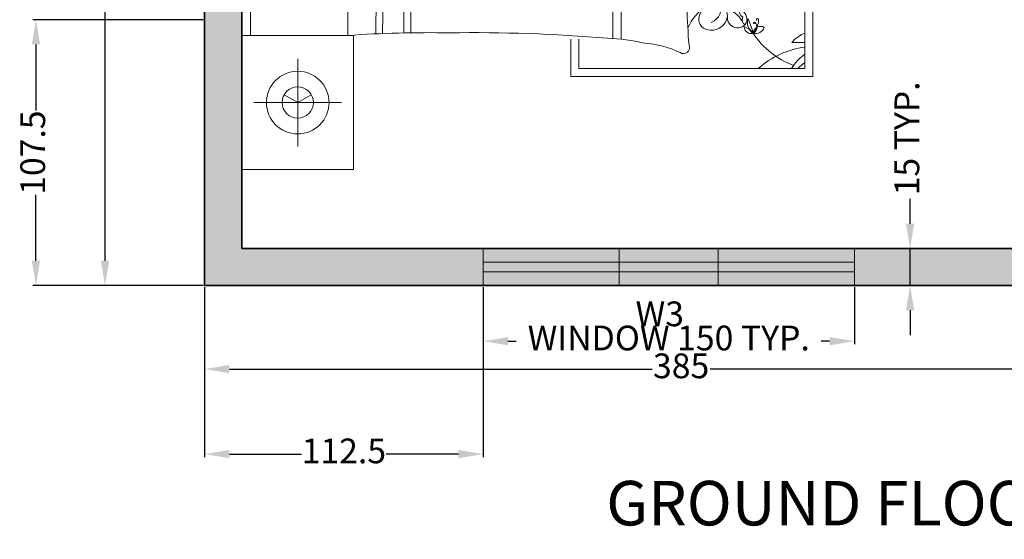
# Model space of a CAD drawing. Units: centimetres. Extents: x 2401 to 3632, y 2122 to 3526.
# Tile 1 of 10: x 2426 to 2824, y 2163 to 2374. Entities that reach past the tile are written whole.
import ezdxf

# ---------------------------------------------------------------- set-up
doc = ezdxf.new("R2010")
doc.units = ezdxf.units.CM
for name, color, linetype, lineweight in [('A-ANNO-DIMS', 9, 'Continuous', 18), ('A-ANNO-TEXT', 9, 'Continuous', 18), ('A-FURN', 9, 'Continuous', 18), ('A-GLAZ', 4, 'Continuous', 18), ('A-WALL', 7, 'Continuous', 35)]:
    doc.layers.add(name, color=color, linetype=linetype, lineweight=lineweight)
doc.layers.add('A-GLAZ-PATT', color=251, linetype='Continuous', lineweight=13, true_color=0x636466)
doc.layers.add('A-WALL-PATT', color=18, linetype='Continuous', lineweight=13, true_color=0x000000)
doc.styles.get("Standard").update_dxf_attribs({"font": 'arial.ttf'})
doc.dimstyles.new('ISO-25', dxfattribs={"dimtxt": 10, "dimasz": 10, "dimexe": 1.25, "dimexo": 0.625, "dimtad": 0, "dimtxsty": 'Standard', "dimcen": 2.5, "dimadec": 0, "dimazin": 0, "dimtfac": 1, "dimtmove": 0, "dimatfit": 3, "dimfxl": 1, "dimarcsym": 0})

# ---------------------------------------------------------------- blocks, each defined once
blk = doc.blocks.new('bed')
for p, q in [((3025.77, 3949.95), (3025.77, 3649.95)), ((3000.77, 3900.35), (3000.77, 3939.55)), ((2981.17, 3919.95), (3020.37, 3919.95)), ((2770.64, 3910.36), (2878.71, 3910.36)), ((2770.64, 3691.65), (2770.64, 3910.36)), ((2774.11, 3906.88), (2774.11, 3695.12)), ((2875.23, 3906.88), (2774.11, 3906.88)), ((2875.23, 3893.39), (2875.23, 3906.88)), ((2878.71, 3910.36), (2878.71, 3893.39)), ((2856.25, 3708.31), (2856.25, 3893.41)), ((2860, 3708.59), (2860, 3893.41)), ((2937.86, 3890.21), (2940.29, 3892.64)), ((2939.08, 3878.06), (2937.86, 3890.21)), ((2940.29, 3892.64), (2953.05, 3881.7)), ((3025.77, 3889.95), (2943.43, 3889.95)), ((2978.36, 3889.95), (2978.36, 3709.95)), ((3021.92, 3709.95), (3021.92, 3889.95)), ((2953.05, 3881.7), (2961.55, 3870.16)), ((2804.53, 3877.32), (2807.92, 3877.98)), ((2937.86, 3862.87), (2939.08, 3878.06)), ((2961.55, 3870.16), (2969.44, 3848.28)), ((2936.04, 3849.5), (2937.86, 3862.87)), ((2826.78, 3739.05), (2826.78, 3860.86)), ((2804.53, 3856.35), (2807.92, 3855.69)), ((2932.4, 3841.6), (2936.04, 3849.5)), ((2969.44, 3848.28), (2978.36, 3815.57)), ((2929.97, 3831.88), (2932.4, 3841.6)), ((2937.86, 3830.66), (2929.97, 3831.88)), ((2955.47, 3823.98), (2937.86, 3830.66)), ((2950.29, 3711.02), (2949.82, 3826.13)), ((2953.37, 3711.03), (2952.92, 3824.95)), ((2978.36, 3807.54), (2955.47, 3823.98)), ((2962.82, 3710.88), (2961.28, 3819.81)), ((2965.89, 3710.76), (2964.4, 3817.57)), ((2804.53, 3745.65), (2807.92, 3746.31)), ((2804.53, 3724.68), (2807.92, 3724.02)), ((2875.23, 3695.12), (2875.23, 3708.35)), ((2878.71, 3708.28), (2878.71, 3691.65)), ((3000.77, 3699.55), (3000.77, 3660.35)), ((2878.71, 3691.65), (2770.64, 3691.65)), ((2774.11, 3695.12), (2875.23, 3695.12)), ((2981.17, 3679.95), (3020.37, 3679.95))]:
    blk.add_line(p, q)
for points in [[(2975.77, 3889.95), (2975.77, 3949.95), (3025.77, 3949.95)], [(3000.77, 3919.95), (2994.7, 3916.45)], [(3000.77, 3919.95), (3006.83, 3916.45)], [(3025.77, 3709.95), (2975.77, 3709.95), (2975.77, 3649.95), (3025.77, 3649.95)], [(3000.77, 3679.95), (2994.7, 3683.45)], [(3000.77, 3679.95), (3006.83, 3683.45)]]:
    blk.add_lwpolyline(points)
for points in [[(2912.82, 3893.27, 0.001242), (2855.9, 3893.41, -0.127202), (2827.53, 3899.43)], [(3018.29, 3872.72, 0.074897), (2998.69, 3872.36, -0.472817)], [(2997.6, 3801.36, 0.14099), (3017.59, 3800.76, 0.235245)], [(2997.6, 3788.55, -0.14099), (3017.59, 3789.15, -0.235245)], [(3018.29, 3727.19, -0.074897), (2998.69, 3727.55, 0.472817)], [(2862.36, 3708.67, 0.056112), (2845.85, 3706.5, 0.095341), (2829.95, 3702.28)]]:
    blk.add_lwpolyline(points, format="xyb")
for centre, radius in [((3000.77, 3919.95), 14), ((3000.77, 3919.95), 7), ((2785.6, 3864.98), 0.764), ((2793.66, 3859.99), 0.764), ((2793.66, 3742.02), 0.764), ((2785.6, 3737.02), 0.764), ((3000.77, 3679.95), 14), ((3000.77, 3679.95), 7)]:
    blk.add_circle(centre, radius)
for centre, radius, start, end in [((2760.03, 3923.26), 23.79, 306.3036, 316.4814), ((2763.59, 3916.39), 19.09, 303.4617, 330.1116), ((2768.83, 3936.05), 39.18, 277.745, 311.8856), ((2764.96, 3869.02), 39.18, 34.3865, 68.5908), ((2827.73, 3896.66), 2.77, 93.98, 207.3412), ((2768, 3905.7), 15.93, 292.5547, 318.9546), ((2776.56, 3949.33), 54.2, 267.4081, 273.6519), ((2514.5, 3864.44), 312.3, 359.3433, 5.6887), ((2796.37, 3886.9), 4.34, 77.7115, 159.0387), ((2794.02, 3891.25), 3.27, 238.4633, 358.2869), ((2804.75, 3884.63), 9.91, 138.8402, 177.9352), ((2798.78, 3888.31), 3.2, 117.6827, 223.7762), ((2798.06, 3887.99), 3.25, 2.9516, 103.728), ((2824.04, 3897.09), 27.41, 192.5173, 207.1824), ((2793.67, 3886.12), 6.19, 345.4653, 54.2343), ((2803, 3894.63), 6.69, 211.3827, 255.2969), ((2815.84, 3882.53), 7.17, 84.9449, 172.8857), ((2816.56, 3884.61), 5.07, 354.4856, 91.0538), ((2932.84, 4167.71), 275.17, 265.8294, 271.553), ((3046.53, 3887.51), 113.22, 177.4519, 191.3392), ((2795.33, 3884.97), 0.487, 177.9352, 11.4834), ((2795.58, 3885.02), 0.236, 11.4834, 127.9409), ((2796.77, 3886.39), 0.424, 223.7762, 159.7183), ((2805.64, 3885.26), 5.62, 175.969, 254.3045), ((2804.28, 3884.18), 4.5, 350.264, 160.8688), ((2799.41, 3885.11), 2.76, 333.9755, 53.2681), ((2814.2, 3893.11), 14.16, 211.2614, 251.7045), ((2818.55, 3879.71), 6.96, 111.5819, 201.4221), ((2805.66, 3897.83), 22.71, 303.6671, 333.2997), ((2798.17, 3879.2), 5.99, 6.1662, 51.5825), ((2817.43, 3883.78), 8.71, 182.3591, 234.0401), ((2812.81, 3886.16), 9.02, 265.2933, 346.921), ((2813.05, 3893.24), 16.1, 236.2883, 266.5076), ((2810.99, 3881.04), 7.46, 209.9085, 343.1337), ((2814.13, 3876.31), 1.86, 167.3041, 285.1471), ((2819.17, 3867.4), 11.57, 122.7011, 126.3445), ((2821.34, 3879.88), 9.56, 199.2822, 299.1751), ((2824.57, 3889.51), 12.43, 238.8218, 279.1554), ((2819.17, 3867.4), 11.57, 55.785, 94.7304), ((2823.47, 3874.11), 3.61, 30.0293, 52.325), ((2789.51, 3870.54), 0.853, 56.8636, 146.9021), ((2801.41, 3872.25), 8.46, 178.3264, 187.1302), ((2792.27, 3871.07), 1.58, 11.3256, 64.4621), ((2797.62, 3873.34), 4.74, 190.2588, 210.656), ((2797.6, 3874.36), 4.82, 218.2101, 226.3071), ((2775.06, 3890.75), 28.48, 313.1541, 322.0459), ((2796.01, 3873.64), 0.586, 142.4737, 265.053), ((2796.78, 3873.76), 1.26, 127.7621, 169.0403), ((2796.11, 3874.82), 1.78, 265.053, 338.3618), ((2798.46, 3872.39), 2.32, 113.4276, 137.6104), ((2798.2, 3874.8), 0.764, 183.2768, 356.7232), ((2798.76, 3873.41), 1.25, 139.7889, 227.6792), ((2798.36, 3872.98), 0.658, 227.6792, 350.3487), ((2795.81, 3873.43), 2.5, 353.0852, 15.7171), ((2797.45, 3873.13), 1.58, 350.3487, 43.6538), ((2800.38, 3874.76), 1.84, 198.7263, 262.5032), ((2798.92, 3873.91), 0.73, 1.1081, 91.8675), ((2800.29, 3873.51), 0.59, 255.2356, 54.9248), ((2799.38, 3873.74), 1.27, 11.5637, 52.6358), ((2816.22, 3868.58), 6.15, 41.5653, 105.1471), ((2819.61, 3881.32), 8.62, 277.436, 299.9149), ((2824.18, 3875.64), 4.49, 221.5653, 293.8354), ((2823.47, 3874.11), 3.61, 314.4517, 333.558), ((3021.8, 3862.02), 40.2, 165.1039, 191.0369), ((2990.83, 3834.5), 38.67, 65.1316, 101.7583), ((5873.3, 3707.37), 2859.79, 176.68521, 177.14978), ((2785.02, 3866.54), 1.51, 157.4086, 261.4386), ((2784.17, 3866.59), 0.757, 58.0499, 135.6268), ((2783.3, 3865.19), 2.41, 14.7558, 58.0499), ((2786.72, 3869.91), 0.853, 124.3538, 214.3923), ((2787.97, 3869.78), 1.99, 190.3057, 287.1958), ((2788.54, 3870.49), 2.31, 176.9701, 248.2913), ((2805.02, 3882.67), 22.32, 212.6784, 216.3746), ((2787.76, 3869.95), 0.883, 216.3746, 291.7548), ((2795.58, 3857.56), 12.46, 124.0033, 132.4917), ((2782.77, 3855.98), 13.31, 63.7819, 68.2913), ((2789.87, 3866.22), 2.12, 128.3208, 208.8162), ((2789.87, 3869.34), 1.99, 122.8155, 187.3992), ((2788.34, 3868.51), 0.666, 289.3605, 111.7548), ((2788.84, 3868.51), 0.666, 221.8703, 44.2646), ((2791.86, 3866.57), 3.48, 157.2305, 229.0635), ((2790.75, 3869.08), 2.31, 109.4799, 177.6828), ((2790.69, 3867.72), 2.05, 174.4544, 220.6188), ((2779.03, 3856.28), 14.94, 30.544, 49.818), ((2789.95, 3869.59), 0.883, 148.8844, 224.2646), ((2808.3, 3858.51), 22.32, 145.1882, 148.8844), ((2795.58, 3857.56), 12.46, 94.756, 119.2041), ((2822.1, 3839.62), 40.99, 132.2412, 142.1744), ((2794.44, 3871.41), 1.44, 188.3432, 274.2869), ((2795.7, 3872.2), 2.51, 210.656, 242.6341), ((2794.04, 3870.31), 0.611, 325.7657, 67.4417), ((2796.2, 3845.18), 24.85, 73.5842, 93.8277), ((2811.5, 3870.46), 8.46, 178.3264, 187.1302), ((2802.37, 3869.29), 1.58, 11.3256, 64.4621), ((2807.71, 3871.55), 4.74, 190.2588, 210.656), ((2804.53, 3869.62), 1.44, 188.3432, 274.2869), ((2805.8, 3870.42), 2.51, 210.656, 242.6341), ((2807.7, 3872.58), 4.82, 218.2101, 226.3071), ((2804.13, 3868.53), 0.611, 325.7657, 67.4417), ((2805.85, 3867.41), 1.44, 147.5332, 233.4768), ((2804.7, 3867.58), 0.611, 354.3784, 96.0543), ((2807.15, 3868.15), 2.51, 179.1859, 211.164), ((2796.2, 3845.18), 24.85, 63.0032, 69.8941), ((2809.96, 3868.8), 4.82, 195.5129, 203.6099), ((2783.42, 3863.83), 0.586, 142.4737, 265.053), ((2784.19, 3863.94), 1.26, 61.2196, 169.0403), ((2783.52, 3865.01), 1.78, 265.053, 338.3618), ((2785.87, 3862.58), 2.32, 113.4276, 137.6104), ((2784.96, 3866.11), 0.506, 172.906, 277.132), ((2786.17, 3863.6), 1.25, 139.7889, 227.6792), ((2785.77, 3863.16), 0.658, 227.6792, 350.3487), ((2786.67, 3865.83), 1.04, 36.1046, 181.4281), ((2783.22, 3863.62), 2.5, 353.0852, 15.7171), ((2784.86, 3863.32), 1.58, 350.3487, 43.6538), ((2787.79, 3864.95), 1.84, 198.7263, 262.5032), ((2786.06, 3866.65), 1.05, 270.0645, 331.1507), ((2786.96, 3866.4), 1.2, 221.8413, 265.7877), ((2786.33, 3864.09), 0.73, 1.1081, 91.8675), ((2786.95, 3865.94), 0.749, 263.7526, 41.7054), ((2786.79, 3863.93), 1.27, 11.5637, 86.365), ((2787.7, 3863.7), 0.59, 255.2356, 54.9248), ((2790.26, 3866.38), 2.53, 207.7043, 254.3516), ((2788.61, 3864.93), 3.48, 270.278, 342.111), ((2790.93, 3860.58), 2.46, 98.7227, 159.3375), ((2787.26, 3864.79), 2.46, 340.0041, 40.6188), ((2790.25, 3865.04), 2.05, 278.7227, 324.8872), ((2789.89, 3863.37), 2.12, 290.5253, 358.5375), ((2794.02, 3863.97), 2.12, 182.8499, 266.1226), ((2793.19, 3865.47), 2.05, 231.7607, 277.9252), ((2794.79, 3865.83), 3.48, 214.5369, 286.3699), ((2793.81, 3861), 2.46, 37.3105, 97.9252), ((2809.06, 3869.3), 4.74, 211.164, 231.5612), ((2809.89, 3873.16), 8.46, 234.6898, 243.4936), ((2804.54, 3865.66), 1.58, 357.3579, 50.4944), ((2811.3, 3865.97), 0.578, 12.7051, 190.4384), ((2811.66, 3866.04), 0.94, 190.4384, 10.4136), ((2821.34, 3853.79), 9.56, 60.8249, 160.7178), ((2911.57, 3860.44), 24.42, 336.2616, 11.3392), ((2789.7, 3863.74), 2.53, 244.9899, 291.6373), ((2791.47, 3858.83), 0.586, 142.4737, 265.053), ((2792.24, 3858.95), 1.26, 61.2196, 169.0403), ((2791.57, 3860.01), 1.78, 265.053, 338.3618), ((2793.07, 3861.54), 1.51, 157.4086, 261.4386), ((2792.22, 3861.59), 0.757, 58.0499, 135.6268), ((2793.92, 3857.58), 2.32, 113.4276, 137.6104), ((2793.01, 3861.12), 0.506, 172.906, 277.132), ((2791.35, 3860.19), 2.41, 14.7558, 58.0499), ((2779.03, 3856.28), 14.94, 23.0501, 23.8477), ((2794.22, 3858.6), 1.25, 139.7889, 227.6792), ((2794.72, 3860.83), 1.04, 36.1046, 181.4281), ((2791.27, 3858.62), 2.5, 353.0852, 15.7171), ((2794.09, 3864.38), 2.53, 265.0106, 311.658), ((2792.91, 3858.32), 1.58, 350.3487, 43.6538), ((2795.84, 3859.95), 1.84, 198.7263, 262.5032), ((2794.11, 3861.65), 1.05, 270.0645, 331.1507), ((2795.01, 3861.4), 1.2, 221.8413, 265.7877), ((2794.38, 3859.1), 0.73, 1.1081, 91.8675), ((2795, 3860.95), 0.749, 263.7526, 41.7054), ((2794.84, 3858.93), 1.27, 11.5637, 86.365), ((2795.75, 3858.7), 0.59, 255.2356, 54.9248), ((2810.99, 3852.63), 7.46, 16.8663, 150.0915), ((2814.13, 3857.35), 1.86, 74.8529, 192.6959), ((2816.22, 3865.09), 6.15, 254.8529, 318.4347), ((2819.61, 3852.35), 8.62, 60.0851, 82.564), ((2824.18, 3858.03), 4.49, 66.1646, 138.4347), ((2823.47, 3859.56), 3.61, 23.229, 45.5483), ((2793.82, 3858.17), 0.658, 227.6792, 350.3487), ((2779.03, 3856.28), 14.94, 357.1071, 4.7585), ((2805.64, 3848.41), 5.62, 105.6955, 184.031), ((2798.17, 3854.46), 5.99, 308.4175, 353.8338), ((2814.2, 3840.56), 14.16, 108.2955, 148.7386), ((2813.05, 3840.43), 16.1, 93.4924, 123.7117), ((2817.43, 3849.89), 8.71, 125.9599, 177.6409), ((2818.55, 3853.96), 6.96, 158.5779, 248.4181), ((2812.81, 3847.51), 9.02, 13.079, 94.7067), ((2819.17, 3866.26), 11.57, 233.6555, 237.2989), ((2824.57, 3844.16), 12.43, 79.7133, 121.1782), ((2819.17, 3866.26), 11.57, 265.2696, 304.215), ((2805.66, 3835.83), 22.71, 21.4941, 56.3329), ((2823.47, 3859.56), 3.61, 307.675, 336.7144), ((3050.38, 3840.86), 69.73, 168.0397, 199.2615), ((2804.28, 3849.49), 4.5, 199.1312, 9.736), ((2799.41, 3848.56), 2.76, 306.7319, 26.0245), ((2815.84, 3851.14), 7.17, 187.1143, 275.0551), ((2816.56, 3849.06), 5.07, 268.9462, 5.5144), ((3043.34, 3811.05), 116.34, 160.1194, 169.3383), ((2909.73, 3831.62), 108.8, 352.2196, 9.497), ((2794.02, 3842.42), 3.27, 1.7131, 121.5367), ((2796.37, 3846.77), 4.34, 200.9613, 282.2885), ((2795.33, 3848.7), 0.487, 348.5166, 182.0648), ((2804.75, 3849.04), 9.91, 182.0648, 221.1598), ((2795.58, 3848.65), 0.236, 232.0591, 348.5166), ((2798.78, 3845.36), 3.2, 136.2238, 242.3173), ((2796.93, 3847.24), 0.255, 200.2667, 136.2271), ((2793.67, 3847.55), 6.19, 305.7657, 14.5347), ((2824.04, 3836.58), 27.41, 152.8176, 167.4827), ((2798.06, 3845.68), 3.25, 256.272, 357.0484), ((2803, 3839.04), 6.69, 104.7031, 148.6173), ((2768, 3827.97), 15.93, 41.0454, 67.4453), ((2764.96, 3864.65), 39.18, 291.4092, 325.6135), ((2776.56, 3784.33), 54.2, 86.3481, 92.5919), ((2768.83, 3797.62), 39.18, 4.4623, 82.255), ((2763.59, 3817.28), 19.09, 1.272, 56.5383), ((2929.73, 3832.56), 0.724, 178.8623, 289.7536), ((2760.03, 3810.41), 23.79, 17.8504, 53.6964), ((2753.34, 3797.91), 35.39, 34.0123, 54.053), ((2747.85, 3800.62), 39.18, 4.4623, 27.4146), ((3035.15, 3812.63), 52.9, 169.8617, 193.6238), ((2964.72, 3808.64), 53.46, 351.5249, 13.96), ((2753.52, 3811.58), 21.54, 343.5431, 17.0202), ((2742.41, 3803.04), 31.85, 4.3787, 5.6357), ((2720.59, 3786.27), 56.92, 19.7217, 19.9028), ((2783.99, 3800.45), 4.34, 47.7873, 129.1145), ((2784.12, 3805.39), 3.27, 208.5391, 328.3627), ((2790.12, 3794.3), 9.91, 108.9159, 148.011), ((2786.78, 3800.47), 3.2, 87.7585, 193.852), ((2813.06, 3795.47), 27.41, 162.593, 177.2582), ((2781.26, 3801.12), 6.19, 315.5411, 24.3101), ((2793.6, 3803.84), 6.69, 181.4585, 225.3727), ((2786, 3800.55), 3.25, 333.0274, 73.8037), ((2804.97, 3797.45), 4.34, 47.7873, 129.1145), ((2987.57, 3836.72), 36.76, 264.0129, 285.8293), ((2782.13, 3799.29), 0.487, 148.011, 341.5592), ((2782.37, 3799.21), 0.236, 341.5592, 98.0167), ((2784.08, 3799.8), 0.424, 193.852, 129.9245), ((2805.11, 3802.39), 3.27, 208.5391, 328.3627), ((2811.1, 3791.3), 9.91, 108.9159, 148.011), ((2807.77, 3797.47), 3.2, 87.7585, 193.852), ((2805.07, 3796.8), 0.424, 193.852, 129.9245), ((2802.25, 3798.12), 6.19, 315.5411, 24.3101), ((2834.04, 3792.47), 27.41, 162.593, 177.2582), ((2802.25, 3793.88), 6.19, 335.6899, 44.4589), ((2834.04, 3799.53), 27.41, 182.7418, 197.407), ((2806.98, 3797.55), 3.25, 333.0274, 73.8037), ((2814.58, 3800.84), 6.69, 181.4585, 225.3727), ((2782.13, 3792.71), 0.487, 18.4408, 211.989), ((2790.12, 3797.71), 9.91, 211.989, 251.0841), ((2782.37, 3792.79), 0.236, 261.9833, 18.4408), ((2786.78, 3791.54), 3.2, 166.148, 272.2415), ((2784.25, 3792.24), 0.255, 230.1909, 166.0209), ((2813.06, 3796.53), 27.41, 182.7418, 197.407), ((2781.26, 3790.88), 6.19, 335.6899, 44.4589), ((2793.6, 3788.16), 6.69, 134.6273, 178.5415), ((2786, 3791.45), 3.25, 286.1963, 26.9726), ((2805.11, 3789.62), 3.27, 31.6373, 151.4609), ((2803.11, 3796.29), 0.487, 148.011, 341.5592), ((2803.11, 3795.71), 0.487, 18.4408, 211.989), ((2811.1, 3800.7), 9.91, 211.989, 251.0841), ((2803.35, 3796.21), 0.236, 341.5592, 98.0167), ((2803.35, 3795.79), 0.236, 261.9833, 18.4408), ((2807.77, 3794.53), 3.2, 166.148, 272.2415), ((2805.23, 3795.24), 0.255, 230.1909, 166.0209), ((2806.98, 3794.45), 3.25, 286.1963, 26.9726), ((2814.58, 3791.16), 6.69, 134.6273, 178.5415), ((2777.88, 3795.65), 30.32, 262.8636, 351.8197), ((2784.12, 3786.62), 3.27, 31.6373, 151.4609), ((2783.99, 3791.55), 4.34, 230.8855, 312.2127), ((2747.85, 3791.38), 39.18, 332.5854, 355.5377), ((2804.97, 3794.55), 4.34, 230.8855, 312.2127), ((2998.15, 3783.03), 15.9, 155.0183, 198.5407), ((2987.57, 3753.18), 36.76, 74.1707, 95.9871), ((3003.33, 3785.03), 14.84, 333.3437, 16.1026), ((2753.52, 3780.42), 21.54, 342.9798, 16.4569), ((2742.41, 3788.96), 31.85, 354.3643, 355.6213), ((2720.59, 3805.74), 56.92, 340.0972, 340.2783), ((2780.65, 3791.73), 17.54, 248.117, 276.6195), ((2775.77, 3775.64), 7.03, 256.3898, 349.0739), ((2776.73, 3780.92), 8.89, 252.8609, 311.9049), ((2764.96, 3737.36), 39.18, 34.3865, 68.5908), ((3018.84, 3755.24), 38.19, 153.8761, 196.1746), ((2965.8, 3762.79), 52.74, 346.3427, 11.1841), ((2776.56, 3817.67), 54.2, 267.4081, 273.6519), ((2768, 3774.04), 15.93, 292.5547, 318.9546), ((2796.37, 3755.24), 4.34, 77.7115, 159.0387), ((2794.02, 3759.58), 3.27, 238.4633, 358.2869), ((2804.75, 3752.96), 9.91, 138.8402, 177.9352), ((2798.78, 3756.64), 3.2, 117.6827, 223.7762), ((2798.06, 3756.33), 3.25, 2.9516, 103.728), ((2803, 3762.97), 6.69, 211.3827, 255.2969), ((2793.67, 3754.46), 6.19, 345.4653, 54.2343), ((2824.04, 3765.42), 27.41, 192.5173, 207.1824), ((2804.28, 3752.51), 4.5, 350.264, 160.8688), ((2815.84, 3750.86), 7.17, 84.9449, 172.8857), ((2816.56, 3752.94), 5.07, 354.4856, 91.0538), ((2805.66, 3766.17), 22.71, 303.6671, 338.5059), ((2795.33, 3753.3), 0.487, 177.9352, 11.4834), ((2795.58, 3753.35), 0.236, 11.4834, 127.9409), ((2796.77, 3754.72), 0.424, 223.7762, 159.7183), ((2805.64, 3753.59), 5.62, 175.969, 254.3045), ((2799.41, 3753.44), 2.76, 333.9755, 53.2681), ((2814.2, 3761.44), 14.16, 211.2614, 251.7045), ((2818.55, 3748.05), 6.96, 111.5819, 201.4221), ((2798.17, 3747.54), 5.99, 6.1662, 51.5825), ((2813.05, 3761.57), 16.1, 236.2883, 266.5076), ((2817.43, 3752.11), 8.71, 182.3591, 234.0401), ((2812.81, 3754.5), 9.02, 265.2933, 346.921), ((5873.3, 3892.54), 2859.79, 182.85022, 183.31479), ((2794.22, 3743.4), 1.25, 132.3208, 220.2111), ((2793.82, 3743.84), 0.658, 9.6513, 132.3208), ((2779.03, 3745.73), 14.94, 355.2415, 2.8929), ((2792.91, 3743.68), 1.58, 316.3462, 9.6513), ((2795.84, 3742.05), 1.84, 97.4968, 161.2737), ((2795.75, 3743.3), 0.59, 305.0752, 104.7644), ((2810.99, 3749.37), 7.46, 209.9085, 343.1337), ((2814.13, 3744.65), 1.86, 167.3041, 285.1471), ((2819.17, 3735.74), 11.57, 122.7011, 126.3445), ((2821.34, 3748.21), 9.56, 199.2822, 299.1751), ((2824.57, 3757.84), 12.43, 238.8218, 280.2867), ((2819.17, 3735.74), 11.57, 55.785, 94.7304), ((2823.47, 3742.45), 3.61, 23.2856, 52.325), ((3021.8, 3737.89), 40.2, 168.9631, 194.8961), ((2785.77, 3738.84), 0.658, 9.6513, 132.3208), ((2789.7, 3738.26), 2.53, 68.3627, 115.0101), ((2788.61, 3737.07), 3.48, 17.889, 89.722), ((2790.93, 3741.42), 2.46, 200.6625, 261.2773), ((2789.89, 3738.63), 2.12, 1.4625, 69.4747), ((2791.47, 3743.17), 0.586, 94.947, 217.5263), ((2792.24, 3743.06), 1.26, 190.9597, 298.7804), ((2791.57, 3741.99), 1.78, 21.6382, 94.947), ((2793.07, 3740.46), 1.51, 98.5614, 202.5914), ((2792.22, 3740.41), 0.757, 224.3732, 301.9501), ((2794.02, 3738.03), 2.12, 93.8774, 177.1501), ((2794.79, 3736.17), 3.48, 73.6301, 145.4631), ((2793.92, 3744.42), 2.32, 222.3896, 246.5724), ((2793.01, 3740.89), 0.506, 82.868, 187.094), ((2791.35, 3741.81), 2.41, 301.9501, 345.2442), ((2779.03, 3745.73), 14.94, 336.1523, 336.9499), ((2793.81, 3741), 2.46, 262.0748, 322.6895), ((2791.27, 3743.38), 2.5, 344.2829, 6.9148), ((2794.72, 3741.17), 1.04, 178.5719, 323.8954), ((2794.09, 3737.62), 2.53, 48.342, 94.9894), ((2795.01, 3740.6), 1.2, 94.2123, 138.1587), ((2794.11, 3740.35), 1.05, 28.8493, 89.9355), ((2794.38, 3742.91), 0.73, 268.1325, 358.8919), ((2794.84, 3743.07), 1.27, 273.635, 348.4363), ((2795, 3741.06), 0.749, 318.2946, 96.2474), ((2816.22, 3736.91), 6.15, 41.5653, 105.1471), ((2819.61, 3749.66), 8.62, 277.436, 299.9149), ((2824.18, 3743.97), 4.49, 221.5653, 293.8354), ((2823.47, 3742.45), 3.61, 314.4517, 336.7144), ((2783.42, 3738.18), 0.586, 94.947, 217.5263), ((2784.19, 3738.06), 1.26, 190.9597, 298.7804), ((2783.52, 3736.99), 1.78, 21.6382, 94.947), ((2785.02, 3735.46), 1.51, 98.5614, 202.5914), ((2785.87, 3739.42), 2.32, 222.3896, 246.5724), ((2784.96, 3735.89), 0.506, 82.868, 187.094), ((2783.3, 3736.82), 2.41, 301.9501, 345.2442), ((2786.17, 3738.4), 1.25, 132.3208, 220.2111), ((2783.22, 3738.38), 2.5, 344.2829, 6.9148), ((2786.67, 3736.18), 1.04, 178.5719, 323.8954), ((2784.86, 3738.68), 1.58, 316.3462, 9.6513), ((2787.79, 3737.05), 1.84, 97.4968, 161.2737), ((2786.96, 3735.61), 1.2, 94.2123, 138.1587), ((2786.06, 3735.36), 1.05, 28.8493, 89.9355), ((2786.33, 3737.91), 0.73, 268.1325, 358.8919), ((2786.79, 3738.08), 1.27, 273.635, 348.4363), ((2786.95, 3736.06), 0.749, 318.2946, 96.2474), ((2795.58, 3744.44), 12.46, 227.5083, 235.9967), ((2787.7, 3738.3), 0.59, 305.0752, 104.7644), ((2789.87, 3735.78), 2.12, 151.1838, 231.6792), ((2790.26, 3735.62), 2.53, 105.6484, 152.2957), ((2791.86, 3735.43), 3.48, 130.9365, 202.7695), ((2790.69, 3734.28), 2.05, 139.3812, 185.5456), ((2779.03, 3745.73), 14.94, 310.182, 329.456), ((2787.26, 3737.22), 2.46, 319.3812, 19.9959), ((2822.1, 3762.38), 40.99, 217.8256, 227.7588), ((2790.25, 3736.96), 2.05, 35.1128, 81.2773), ((2793.19, 3736.53), 2.05, 82.0748, 128.2393), ((2805.85, 3734.59), 1.44, 126.5232, 212.4668), ((2807.15, 3733.85), 2.51, 148.836, 180.8141), ((2809.06, 3732.7), 4.74, 128.4388, 148.836), ((2809.89, 3728.84), 8.46, 116.5064, 125.3102), ((2809.96, 3733.2), 4.82, 156.3901, 164.4871), ((2804.54, 3736.34), 1.58, 309.5056, 2.6421), ((2811.3, 3736.03), 0.578, 169.5616, 347.2949), ((2811.66, 3735.96), 0.94, 349.5864, 169.5616), ((2535.01, 3729.86), 291.92, 355.2402, 1.8035), ((2784.17, 3735.41), 0.757, 224.3732, 301.9501), ((2786.72, 3732.09), 0.853, 145.6077, 235.6462), ((2787.97, 3732.22), 1.99, 72.8042, 169.6943), ((2788.54, 3731.51), 2.31, 111.7087, 183.0299), ((2805.02, 3719.34), 22.32, 143.6254, 147.3216), ((2787.76, 3732.05), 0.883, 68.2452, 143.6254), ((2782.77, 3746.02), 13.31, 291.7087, 296.2181), ((2789.87, 3732.67), 1.99, 172.6008, 237.1845), ((2788.34, 3733.49), 0.666, 248.2452, 70.6395), ((2788.84, 3733.49), 0.666, 315.7354, 138.1297), ((2790.75, 3732.92), 2.31, 182.3172, 250.5201), ((2789.51, 3731.46), 0.853, 213.0979, 303.1364), ((2789.95, 3732.41), 0.883, 135.7354, 211.1156), ((2808.3, 3743.49), 22.32, 211.1156, 214.8118), ((2795.58, 3744.44), 12.46, 240.7959, 265.244), ((2797.62, 3728.66), 4.74, 149.344, 169.7412), ((2801.41, 3729.75), 8.46, 172.8698, 181.6736), ((2792.27, 3730.93), 1.58, 295.5379, 348.6744), ((2794.44, 3730.6), 1.44, 85.7131, 171.6568), ((2795.7, 3729.8), 2.51, 117.3659, 149.344), ((2797.6, 3727.64), 4.82, 133.6929, 141.7899), ((2794.04, 3731.69), 0.611, 292.5583, 34.2343), ((2796.2, 3756.82), 24.85, 266.1723, 286.4158), ((2775.06, 3711.25), 28.48, 37.9541, 46.8459), ((2811.5, 3731.54), 8.46, 172.8698, 181.6736), ((2807.71, 3730.45), 4.74, 149.344, 169.7412), ((2802.37, 3732.72), 1.58, 295.5379, 348.6744), ((2804.53, 3732.38), 1.44, 85.7131, 171.6568), ((2805.8, 3731.59), 2.51, 117.3659, 149.344), ((2807.7, 3729.43), 4.82, 133.6929, 141.7899), ((2804.13, 3733.47), 0.611, 292.5583, 34.2343), ((2804.7, 3734.43), 0.611, 263.9457, 5.6216), ((2796.2, 3756.82), 24.85, 290.1059, 296.9968), ((2821.34, 3722.12), 9.56, 60.8249, 160.7178), ((2824.18, 3726.36), 4.49, 66.1646, 138.4347), ((2796.01, 3728.36), 0.586, 94.947, 217.5263), ((2796.78, 3728.25), 1.26, 190.9597, 232.2379), ((2796.11, 3727.18), 1.78, 21.6382, 94.947), ((2798.46, 3729.61), 2.32, 222.3896, 246.5724), ((2798.2, 3727.21), 0.764, 3.2768, 176.7232), ((2798.76, 3728.59), 1.25, 132.3208, 220.2111), ((2798.36, 3729.03), 0.658, 9.6513, 132.3208), ((2795.81, 3728.57), 2.5, 344.2829, 6.9148), ((2797.45, 3728.87), 1.58, 316.3462, 9.6513), ((2800.38, 3727.24), 1.84, 97.4968, 161.2737), ((2798.92, 3728.1), 0.73, 268.1325, 358.8919), ((2800.29, 3728.49), 0.59, 305.0752, 104.7644), ((2799.38, 3728.26), 1.27, 307.3642, 348.4363), ((2810.99, 3720.97), 7.46, 16.8663, 150.0915), ((2814.13, 3725.69), 1.86, 74.8529, 192.6959), ((2816.22, 3733.42), 6.15, 254.8529, 318.4347), ((2819.61, 3720.68), 8.62, 60.0851, 82.564), ((2823.47, 3727.89), 3.61, 307.675, 342.5814), ((2823.47, 3727.89), 3.61, 16.6343, 45.5483), ((2990.83, 3765.41), 38.67, 258.2417, 294.8684), ((2805.64, 3716.74), 5.62, 105.6955, 184.031), ((2798.17, 3722.8), 5.99, 308.4175, 353.8338), ((2814.2, 3708.9), 14.16, 108.2955, 148.7386), ((2813.05, 3708.76), 16.1, 93.4924, 123.7117), ((2817.43, 3718.23), 8.71, 125.9599, 177.6409), ((2818.55, 3722.29), 6.96, 158.5779, 248.4181), ((2812.81, 3715.84), 9.02, 13.079, 94.7067), ((2819.17, 3734.6), 11.57, 233.6555, 237.2989), ((2824.57, 3712.5), 12.43, 79.249, 121.1782), ((2819.17, 3734.6), 11.57, 265.2696, 304.215), ((2805.66, 3704.17), 22.71, 23.6453, 56.3329), ((2795.33, 3717.04), 0.487, 348.5166, 182.0648), ((2824.04, 3704.91), 27.41, 152.8176, 167.4827), ((2793.67, 3715.88), 6.19, 305.7657, 14.5347), ((2804.28, 3717.82), 4.5, 199.1312, 9.736), ((2799.41, 3716.9), 2.76, 306.7319, 26.0245), ((2815.84, 3719.47), 7.17, 187.1143, 275.0551), ((2816.56, 3717.4), 5.07, 268.9462, 5.5144), ((2794.02, 3710.76), 3.27, 1.7131, 121.5367), ((2796.37, 3715.1), 4.34, 200.9613, 282.2885), ((2804.75, 3717.37), 9.91, 182.0648, 221.1598), ((2795.58, 3716.99), 0.236, 232.0591, 348.5166), ((2798.78, 3713.69), 3.2, 136.2238, 242.3173), ((2796.93, 3715.57), 0.255, 200.2667, 136.2271), ((2803, 3707.37), 6.69, 104.7031, 148.6173), ((2798.06, 3714.01), 3.25, 256.272, 357.0484), ((2768, 3696.3), 15.93, 41.0454, 67.4453), ((2764.96, 3732.98), 39.18, 291.4092, 325.6135), ((2922.1, 3008.05), 703.17, 89.11454, 94.87351), ((2941.69, 3172.15), 539.05, 86.1, 90.9282), ((2776.56, 3652.67), 54.2, 86.3481, 92.5919), ((2768.83, 3665.96), 39.18, 48.1144, 82.255), ((2828.43, 3704.55), 2.73, 156.5219, 303.8264), ((2763.59, 3685.61), 19.09, 29.8884, 56.5383), ((2760.03, 3678.74), 23.79, 43.5186, 53.6964)]:
    blk.add_arc(centre, radius, start, end)
blk = doc.blocks.new('*D12')
at = {"layer": 'A-ANNO-DIMS', "color": 0, "lineweight": -2, "transparency": 16777216}
for p, q in [((2499.81, 3451.1), (2458.94, 3451.1)), ((2460.19, 3441.1), (2460.19, 2873.73)), ((2460.19, 2276.1), (2460.19, 2843.48)), ((2499.81, 2266.1), (2458.94, 2266.1))]:
    blk.add_line(p, q, dxfattribs=at)
at = {"layer": 'A-ANNO-DIMS', "color": 0, "transparency": 16777216}
for points in [[(2458.52, 3441.1), (2461.85, 3441.1), (2460.19, 3451.1)], [(2458.52, 2276.1), (2461.85, 2276.1), (2460.19, 2266.1)]]:
    blk.add_solid(points, dxfattribs=at)
at = {"layer": 'Defpoints', "color": 0, "transparency": 16777216}
for p in [(2500.44, 3451.1), (2460.19, 2266.1), (2500.44, 2266.1)]:
    blk.add_point(p, dxfattribs=at)
at = {"layer": 'A-ANNO-DIMS', "color": 0, "transparency": 16777216, "insert": (2460.19, 2858.6), "char_height": 10, "attachment_point": 5, "rotation": 90}
blk.add_mtext('1185', dxfattribs=at)
blk = doc.blocks.new('*D13')
at = {"layer": 'A-ANNO-DIMS', "color": 0, "lineweight": -2, "transparency": 16777216}
for p, q in [((2500.44, 2265.48), (2500.44, 2231.09)), ((2885.44, 2265.48), (2885.44, 2231.09)), ((2510.44, 2232.34), (2681.23, 2232.34)), ((2875.44, 2232.34), (2704.64, 2232.34))]:
    blk.add_line(p, q, dxfattribs=at)
at = {"layer": 'A-ANNO-DIMS', "color": 0, "transparency": 16777216}
for points in [[(2510.44, 2234.01), (2510.44, 2230.67), (2500.44, 2232.34)], [(2875.44, 2234.01), (2875.44, 2230.67), (2885.44, 2232.34)]]:
    blk.add_solid(points, dxfattribs=at)
at = {"layer": 'Defpoints', "color": 0, "transparency": 16777216}
for p in [(2500.44, 2266.1), (2885.44, 2266.1), (2885.44, 2232.34)]:
    blk.add_point(p, dxfattribs=at)
at = {"layer": 'A-ANNO-DIMS', "color": 0, "transparency": 16777216, "insert": (2692.94, 2232.34), "char_height": 10, "attachment_point": 5}
blk.add_mtext('385', dxfattribs=at)
blk = doc.blocks.new('WIN-1500-3P')
for p, q in [((0, 15), (0, 0)), ((55, 15), (55, 0)), ((95, 15), (95, 0)), ((150, 15), (150, 0)), ((0, 9.5), (150, 9.5)), ((0, 5.5), (150, 5.5))]:
    blk.add_line(p, q)
blk = doc.blocks.new('*D20')
at = {"layer": 'A-ANNO-DIMS', "color": 0, "lineweight": -2, "transparency": 16777216}
for p, q in [((2612.94, 2265.48), (2612.94, 2242.35)), ((2762.94, 2265.48), (2762.94, 2242.35)), ((2622.94, 2243.6), (2626.29, 2243.6)), ((2752.94, 2243.6), (2749.58, 2243.6))]:
    blk.add_line(p, q, dxfattribs=at)
at = {"layer": 'A-ANNO-DIMS', "color": 0, "transparency": 16777216}
for points in [[(2622.94, 2245.27), (2622.94, 2241.94), (2612.94, 2243.6)], [(2752.94, 2245.27), (2752.94, 2241.94), (2762.94, 2243.6)]]:
    blk.add_solid(points, dxfattribs=at)
at = {"layer": 'Defpoints', "color": 0, "transparency": 16777216}
for p in [(2612.94, 2266.1), (2762.94, 2266.1), (2762.94, 2243.6)]:
    blk.add_point(p, dxfattribs=at)
at = {"layer": 'A-ANNO-DIMS', "color": 0, "transparency": 16777216, "insert": (2687.94, 2243.6), "char_height": 10, "attachment_point": 5}
blk.add_mtext('WINDOW 150 TYP.', dxfattribs=at)
blk = doc.blocks.new('*D21')
at = {"layer": 'A-ANNO-DIMS', "color": 0, "lineweight": -2, "transparency": 16777216}
for p, q in [((2785.44, 2291.1), (2785.44, 2301.1)), ((2763.56, 2281.1), (2786.69, 2281.1)), ((2785.44, 2266.1), (2785.44, 2281.1)), ((2763.56, 2266.1), (2786.69, 2266.1)), ((2785.44, 2256.1), (2785.44, 2246.1))]:
    blk.add_line(p, q, dxfattribs=at)
at = {"layer": 'A-ANNO-DIMS', "color": 0, "transparency": 16777216}
for points in [[(2783.77, 2291.1), (2787.1, 2291.1), (2785.44, 2281.1)], [(2783.77, 2256.1), (2787.1, 2256.1), (2785.44, 2266.1)]]:
    blk.add_solid(points, dxfattribs=at)
at = {"layer": 'Defpoints', "color": 0, "transparency": 16777216}
for p in [(2762.94, 2281.1), (2785.44, 2281.1), (2762.94, 2266.1)]:
    blk.add_point(p, dxfattribs=at)
at = {"layer": 'A-ANNO-DIMS', "color": 0, "transparency": 16777216, "insert": (2785.44, 2325.6), "char_height": 10, "attachment_point": 5, "rotation": 90}
blk.add_mtext('15 TYP.', dxfattribs=at)
blk = doc.blocks.new('*D38')
at = {"layer": 'A-ANNO-DIMS', "color": 0, "lineweight": -2, "transparency": 16777216}
for p, q in [((2500.44, 2265.48), (2500.44, 2196.7)), ((2612.94, 2265.48), (2612.94, 2196.7)), ((2510.44, 2197.95), (2539.62, 2197.95)), ((2602.94, 2197.95), (2573.75, 2197.95))]:
    blk.add_line(p, q, dxfattribs=at)
at = {"layer": 'A-ANNO-DIMS', "color": 0, "transparency": 16777216}
for points in [[(2510.44, 2199.62), (2510.44, 2196.29), (2500.44, 2197.95)], [(2602.94, 2199.62), (2602.94, 2196.29), (2612.94, 2197.95)]]:
    blk.add_solid(points, dxfattribs=at)
at = {"layer": 'Defpoints', "color": 0, "transparency": 16777216}
for p in [(2500.44, 2266.1), (2612.94, 2266.1), (2612.94, 2197.95)]:
    blk.add_point(p, dxfattribs=at)
at = {"layer": 'A-ANNO-DIMS', "color": 0, "transparency": 16777216, "insert": (2556.69, 2197.95), "char_height": 10, "attachment_point": 5}
blk.add_mtext('112.5', dxfattribs=at)
blk = doc.blocks.new('*D39')
at = {"layer": 'A-ANNO-DIMS', "color": 0, "lineweight": -2, "transparency": 16777216}
for p, q in [((2499.81, 2373.6), (2431.04, 2373.6)), ((2432.29, 2363.6), (2432.29, 2336.92)), ((2432.29, 2276.1), (2432.29, 2302.79)), ((2499.81, 2266.1), (2431.04, 2266.1))]:
    blk.add_line(p, q, dxfattribs=at)
at = {"layer": 'A-ANNO-DIMS', "color": 0, "transparency": 16777216}
for points in [[(2430.62, 2363.6), (2433.95, 2363.6), (2432.29, 2373.6)], [(2430.62, 2276.1), (2433.95, 2276.1), (2432.29, 2266.1)]]:
    blk.add_solid(points, dxfattribs=at)
at = {"layer": 'Defpoints', "color": 0, "transparency": 16777216}
for p in [(2432.29, 2373.6), (2500.44, 2373.6), (2500.44, 2266.1)]:
    blk.add_point(p, dxfattribs=at)
at = {"layer": 'A-ANNO-DIMS', "color": 0, "transparency": 16777216, "insert": (2432.29, 2319.85), "char_height": 10, "attachment_point": 5, "rotation": 90}
blk.add_mtext('107.5', dxfattribs=at)

msp = doc.modelspace()

# ---------------------------------------------------------------- hatches: boundary and pattern name
at = {"layer": 'A-GLAZ-PATT'}
h = msp.add_hatch(color=256, dxfattribs=at)
h.dxf.hatch_style = 1
h.paths.add_polyline_path([(3132.936, 2596.604), (3092.936, 2596.604), (3092.936, 2591.104), (3132.936, 2591.104)])
h.paths.add_polyline_path([(2762.936, 2281.104), (2707.936, 2281.104), (2707.936, 2275.604), (2762.936, 2275.604)])
h.paths.add_polyline_path([(2707.936, 2271.604), (2667.936, 2271.604), (2667.936, 2266.104), (2707.936, 2266.104)])
h.paths.add_polyline_path([(2762.936, 2275.604), (2707.936, 2275.604), (2707.936, 2271.604), (2762.936, 2271.604)])
h.paths.add_polyline_path([(2762.936, 2271.604), (2707.936, 2271.604), (2707.936, 2266.104), (2762.936, 2266.104)])
h.paths.add_polyline_path([(2707.936, 2275.604), (2667.936, 2275.604), (2667.936, 2271.604), (2707.936, 2271.604)])
h.paths.add_polyline_path([(2707.936, 2281.104), (2667.936, 2281.104), (2667.936, 2275.604), (2707.936, 2275.604)])
h.paths.add_polyline_path([(2667.936, 2281.104), (2612.936, 2281.104), (2612.936, 2275.604), (2667.936, 2275.604)])
h.paths.add_polyline_path([(2667.936, 2275.604), (2612.936, 2275.604), (2612.936, 2271.604), (2667.936, 2271.604)])
h.paths.add_polyline_path([(2667.936, 2271.604), (2612.936, 2271.604), (2612.936, 2266.104), (2667.936, 2266.104)])
h.paths.add_polyline_path([(2515.436, 2523.604), (2509.936, 2523.604), (2509.936, 2468.604), (2515.436, 2468.604)])
h.paths.add_polyline_path([(2509.936, 2523.604), (2505.936, 2523.604), (2505.936, 2468.604), (2509.936, 2468.604)])
h.paths.add_polyline_path([(2505.936, 2523.604), (2500.436, 2523.604), (2500.436, 2468.604), (2505.936, 2468.604)])
h.paths.add_polyline_path([(2505.936, 2468.604), (2500.436, 2468.604), (2500.436, 2428.604), (2505.936, 2428.604)])
h.paths.add_polyline_path([(2509.936, 2468.604), (2505.936, 2468.604), (2505.936, 2428.604), (2509.936, 2428.604)])
h.paths.add_polyline_path([(2515.436, 2468.604), (2509.936, 2468.604), (2509.936, 2428.604), (2515.436, 2428.604)])
h.paths.add_polyline_path([(2515.436, 2428.604), (2509.936, 2428.604), (2509.936, 2373.604), (2515.436, 2373.604)])
h.paths.add_polyline_path([(2509.936, 2428.604), (2505.936, 2428.604), (2505.936, 2373.604), (2509.936, 2373.604)])
h.paths.add_polyline_path([(2505.936, 2428.604), (2500.436, 2428.604), (2500.436, 2373.604), (2505.936, 2373.604)])
h.paths.add_polyline_path([(2505.936, 3028.604), (2500.436, 3028.604), (2500.436, 2973.604), (2505.936, 2973.604)])
h.paths.add_polyline_path([(2515.436, 3028.604), (2509.936, 3028.604), (2509.936, 2973.604), (2515.436, 2973.604)])
h.paths.add_polyline_path([(2509.936, 3028.604), (2505.936, 3028.604), (2505.936, 2973.604), (2509.936, 2973.604)])
h.paths.add_polyline_path([(2515.436, 2973.604), (2509.936, 2973.604), (2509.936, 2933.604), (2515.436, 2933.604)])
h.paths.add_polyline_path([(2509.936, 2973.604), (2505.936, 2973.604), (2505.936, 2933.604), (2509.936, 2933.604)])
h.paths.add_polyline_path([(2505.936, 2973.604), (2500.436, 2973.604), (2500.436, 2933.604), (2505.936, 2933.604)])
h.paths.add_polyline_path([(2505.936, 2933.604), (2500.436, 2933.604), (2500.436, 2878.604), (2505.936, 2878.604)])
h.paths.add_polyline_path([(2515.436, 2933.604), (2509.936, 2933.604), (2509.936, 2878.604), (2515.436, 2878.604)])
h.paths.add_polyline_path([(2509.936, 2933.604), (2505.936, 2933.604), (2505.936, 2878.604), (2509.936, 2878.604)])
at = {"layer": 'A-WALL-PATT'}
h = msp.add_hatch(color=256, dxfattribs=at)
h.dxf.hatch_style = 1
h.paths.add_polyline_path([(2765.436, 3451.104), (2500.436, 3451.104), (2500.436, 3356.104), (2515.436, 3356.104), (2515.436, 3436.104), (2765.436, 3436.104)])
h.paths.add_polyline_path([(3245.436, 3451.104), (3127.936, 3451.104), (3127.936, 3436.104), (3185.226, 3436.104), (3185.226, 3436.735), (3230.436, 3436.735), (3230.436, 3356.104), (3245.436, 3356.104)])
h.paths.add_polyline_path([(3245.436, 2686.104), (3230.436, 2686.104), (3230.436, 2606.104), (3187.936, 2606.104), (3187.936, 2591.104), (3245.436, 2591.104)])
h.paths.add_polyline_path([(3037.936, 2606.104), (2995.436, 2606.104), (2995.436, 2591.104), (3037.936, 2591.104)])
h.paths.add_polyline_path([(3245.436, 2976.104), (3230.436, 2976.104), (3230.436, 2931.104), (2980.436, 2931.104), (2980.436, 3096.104), (2965.436, 3096.104), (2965.436, 2916.104), (3230.436, 2916.104), (3230.436, 2836.104), (3245.436, 2836.104)])
h.paths.add_polyline_path([(3230.436, 3096.104), (3055.436, 3096.104), (3055.436, 3081.104), (3230.436, 3081.104)], flags=17)
h.paths.add_polyline_path([(2977.936, 3451.104), (2860.436, 3451.104), (2860.436, 3096.104), (2875.436, 3096.104), (2875.436, 3436.104), (2977.936, 3436.104)])
h.paths.add_polyline_path([(2765.436, 3126.104), (2515.436, 3126.104), (2515.436, 3206.104), (2500.436, 3206.104), (2500.436, 3028.604), (2515.436, 3028.604), (2515.436, 3111.104), (2765.436, 3111.104)])
h.paths.add_polyline_path([(2780.436, 2796.104), (2515.436, 2796.104), (2515.436, 2878.604), (2500.436, 2878.604), (2500.436, 2736.104), (2515.436, 2736.104), (2515.436, 2781.104), (2765.436, 2781.104), (2765.436, 2706.104), (2780.436, 2706.104)])
h.paths.add_polyline_path([(2780.436, 2631.104), (2515.436, 2631.104), (2515.436, 2676.104), (2500.436, 2676.104), (2500.436, 2523.604), (2515.436, 2523.604), (2515.436, 2616.104), (2780.436, 2616.104)])
h.paths.add_polyline_path([(2885.436, 2796.104), (2870.436, 2796.104), (2870.436, 2281.104), (2762.936, 2281.104), (2762.936, 2266.104), (2885.436, 2266.104)])
h.paths.add_polyline_path([(2612.936, 2281.104), (2515.436, 2281.104), (2515.436, 2373.604), (2500.436, 2373.604), (2500.436, 2266.104), (2612.936, 2266.104)])

# ---------------------------------------------------------------- linework, layer by layer
at = {"layer": 'A-WALL'}
for p, q in [((2515.436, 2616.104), (2515.436, 2281.104)), ((2515.436, 2281.104), (2870.436, 2281.104))]:
    msp.add_line(p, q, dxfattribs=at)
msp.add_lwpolyline([(2765.436, 3451.104), (2500.436, 3451.104), (2500.436, 2266.104), (2885.436, 2266.104), (2885.436, 2796.104)], dxfattribs=at)

# ---------------------------------------------------------------- block references
at = {"layer": 'A-FURN', "xscale": -0.9042027756184401, "yscale": 0.9042027756184401, "zscale": 0.9042027756184401}
msp.add_blockref('bed', (5251.343, -987.325), dxfattribs=at)
at = {"layer": 'A-GLAZ'}
msp.add_blockref('WIN-1500-3P', (2612.936, 2266.104), dxfattribs=at)

# ---------------------------------------------------------------- texts
at = {"layer": 'A-ANNO-TEXT', "attachment_point": 1}
for s, width, insert, char_height in [('\\pxqc;W3', 66.28614, (2651.176, 2259.663), 10), ('\\pxqc;{\\fCalifornian FB|b1|i0|c0|p18;GROUND FLOOR PLAN - 83.10 Sq.M  (894.48 SQF)}', 622.58197, (2627.432, 2187.118), 18)]:
    msp.add_mtext_dynamic_manual_height_columns(s, width=width, gutter_width=12.5, heights=[0], dxfattribs=dict(at, insert=insert, char_height=char_height))

# ---------------------------------------------------------------- dimensions: what is measured, and where the dimension line sits
at = {"layer": 'A-ANNO-DIMS'}
for base, p1, p2, override, picture, middle in [((2460.187, 2266.104), (2500.436, 3451.104), (2500.436, 2266.104), {"dimclrd": 0, "dimclre": 0, "dimclrt": 0}, '*D12', (2460.187, 2858.604)), ((2432.286, 2373.604), (2500.436, 2266.104), (2500.436, 2373.604), {"dimdec": 1, "dimlfac": 1, "dimrnd": 0, "dimzin": 0, "dimdsep": 46, "dimlunit": 2}, '*D39', (2432.286, 2319.854))]:
    dim = msp.add_linear_dim(base=base, p1=p1, p2=p2, angle=90, dimstyle='ISO-25', override=override, dxfattribs=at)
    dim.commit()
    dim.dimension.update_dxf_attribs({"geometry": picture, "text_midpoint": middle})
dim = msp.add_linear_dim(base=(2785.436, 2281.104), p1=(2762.936, 2266.104), p2=(2762.936, 2281.104), angle=90, text='<> TYP.', dimstyle='ISO-25', override={"dimdec": 0, "dimlfac": 1, "dimrnd": 0, "dimzin": 0, "dimdsep": 46, "dimlunit": 2}, dxfattribs=at)
dim.commit()
dim.dimension.update_dxf_attribs({"geometry": '*D21', "text_midpoint": (2785.436, 2325.597)})
for base, p2, override, picture, middle in [((2885.436, 2232.34), (2885.436, 2266.104), {"dimclrd": 0, "dimclre": 0, "dimclrt": 0}, '*D13', (2692.936, 2232.34)), ((2612.936, 2197.954), (2612.936, 2266.104), {"dimdec": 1, "dimlfac": 1, "dimrnd": 0, "dimzin": 0, "dimdsep": 46, "dimlunit": 2}, '*D38', (2556.686, 2197.954))]:
    dim = msp.add_linear_dim(base=base, p1=(2500.436, 2266.104), p2=p2, dimstyle='ISO-25', override=override, dxfattribs=at)
    dim.commit()
    dim.dimension.update_dxf_attribs({"geometry": picture, "text_midpoint": middle})
dim = msp.add_linear_dim(base=(2762.936, 2243.604), p1=(2612.936, 2266.104), p2=(2762.936, 2266.104), text='WINDOW <> TYP.', dimstyle='ISO-25', override={"dimdec": 0, "dimlfac": 1, "dimrnd": 0, "dimzin": 0, "dimdsep": 46, "dimlunit": 2}, dxfattribs=at)
dim.commit()
dim.dimension.update_dxf_attribs({"geometry": '*D20', "text_midpoint": (2687.936, 2243.604)})

doc.saveas('drawing.dxf')
